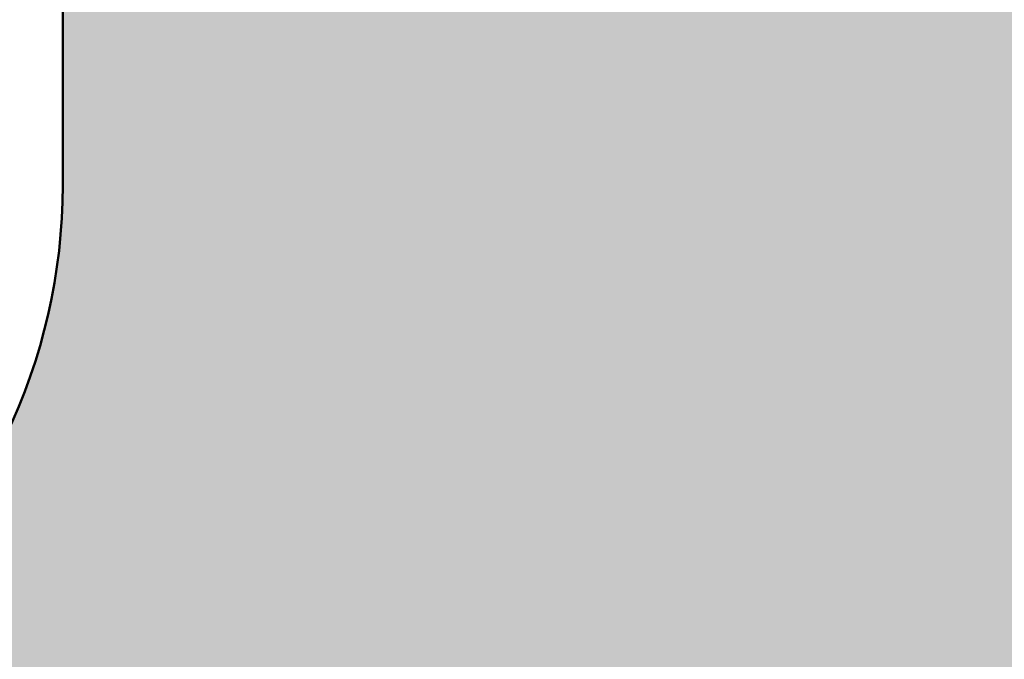
# Model space of a CAD drawing. Units: millimetres. Extents: x 0 to 2267, y 0 to 1823.
# Tile 28 of 256: x 1590 to 1675, y 1160 to 1216. Entities that reach past the tile are written whole.
import ezdxf

# ---------------------------------------------------------------- set-up
doc = ezdxf.new("R2010")
doc.units = ezdxf.units.MM
doc.header["$MEASUREMENT"] = 0
doc.layers.add('M-HATC', color=252, linetype='Continuous', lineweight=18)
doc.layers.add('M-OUTL', color=7, linetype='Continuous', lineweight=50)

msp = doc.modelspace()

# ---------------------------------------------------------------- hatches: boundary and pattern name
at = {"layer": 'M-HATC'}
h = msp.add_hatch(color=256, dxfattribs=at)
h.dxf.hatch_style = 1
h.paths.add_polyline_path([(2055.771, 1603.062), (1381.087, 1603.062), (1381.087, 1598.062), (2055.771, 1598.062)])
h.paths.add_polyline_path([(2055.771, 1598.062), (1381.087, 1598.062), (1381.087, 1593.062), (2055.771, 1593.062)])
h.paths.add_polyline_path([(2051.307, 1536.761), (1385.55, 1536.761), (1385.55, 1526.761), (1387.55, 1526.761), (1388.537, 1525.053), (1385.332, 1521.233), (1385.332, 1521.223), (2050.254, 1522.749), (2048.321, 1525.053), (2049.307, 1526.761), (2051.307, 1526.761)])
edge = h.paths.add_edge_path()
edge.add_arc((1847.535, 1379.149), 135, 222.60306, 222.89085, ccw=False)
edge.add_line((1748.166, 1287.766), (1683.092, 1287.766))
edge.add_arc((1583.724, 1379.149), 135, 317.10915, 317.39694, ccw=False)
edge.add_arc((1678.969, 1290.671), 5, 222.89085, 317.10915, ccw=False)
edge.add_arc((1774.213, 1379.149), 135, 222.60306, 222.89085, ccw=False)
edge.add_line((1674.845, 1287.766), (1609.771, 1287.766))
edge.add_arc((1510.403, 1379.149), 135, 317.10915, 317.39694, ccw=False)
edge.add_arc((1605.647, 1290.671), 5, 222.89085, 317.10915, ccw=False)
edge.add_arc((1700.892, 1379.149), 135, 222.60306, 222.89085, ccw=False)
edge.add_line((1601.524, 1287.766), (1536.45, 1287.766))
edge.add_arc((1437.081, 1379.149), 135, 317.10915, 317.39694, ccw=False)
edge.add_arc((1532.326, 1290.671), 5, 222.89085, 317.10915, ccw=False)
edge.add_arc((1627.571, 1379.149), 135, 222.60306, 222.89085, ccw=False)
edge.add_line((1528.203, 1287.766), (1505.929, 1287.766))
edge.add_spline(control_points=[(1505.929, 1287.766), (1504.262, 1287.766), (1504.262, 1282.766), (1505.929, 1282.766)], knot_values=[0, 0, 0, 0, 5, 5, 5, 5], degree=3, periodic=0)
edge.add_line((1505.929, 1282.766), (1930.929, 1282.766))
edge.add_spline(control_points=[(1930.929, 1282.766), (1932.596, 1282.766), (1932.596, 1287.766), (1930.929, 1287.766)], knot_values=[0, 0, 0, 0, 5, 5, 5, 5], degree=3, periodic=0)
edge.add_line((1930.929, 1287.766), (1903.056, 1287.766))
edge.add_arc((1803.688, 1379.149), 135, 317.10915, 317.39694, ccw=False)
edge.add_arc((1898.932, 1290.671), 5, 222.89085, 317.10915, ccw=False)
edge.add_arc((1994.177, 1379.149), 135, 222.60306, 222.89085, ccw=False)
edge.add_line((1894.809, 1287.766), (1829.735, 1287.766))
edge.add_arc((1730.366, 1379.149), 135, 317.10915, 317.39694, ccw=False)
edge.add_arc((1825.611, 1290.671), 5, 222.89085, 317.10915, ccw=False)
edge.add_arc((1920.856, 1379.149), 135, 222.60306, 222.89085, ccw=False)
edge.add_line((1821.487, 1287.766), (1756.413, 1287.766))
edge.add_arc((1657.045, 1379.149), 135, 317.10915, 317.39694, ccw=False)
edge.add_arc((1752.29, 1290.671), 5, 222.89085, 317.10915, ccw=False)
edge = h.paths.add_edge_path()
edge.add_spline(control_points=[(1843.429, 1227.247), (1845.096, 1227.247), (1845.096, 1232.247), (1843.429, 1232.247)], knot_values=[0, 0, 0, 0, 5, 5, 5, 5], degree=3, periodic=0)
edge.add_line((1843.429, 1232.247), (1593.429, 1232.247))
edge.add_spline(control_points=[(1593.429, 1232.247), (1591.762, 1232.247), (1591.762, 1227.247), (1593.429, 1227.247)], knot_values=[0, 0, 0, 0, 5, 5, 5, 5], degree=3, periodic=0)
edge.add_line((1593.429, 1227.247), (1843.429, 1227.247))
h.paths.add_polyline_path([(1905.929, 1127.417), (1530.929, 1127.417, 0.414214), (1520.929, 1117.417), (1530.929, 1117.417), (1915.929, 1117.417, 0.414214)])
edge = h.paths.add_edge_path()
edge.add_arc((1397.086, 1498.408), 12.73, 90.78215, 190.87871, ccw=False)
edge.add_line((1396.912, 1511.136), (1428.01, 1511.349))
edge.add_line((1428.01, 1511.349), (1433.01, 1511.349))
edge.add_line((1433.01, 1511.349), (1434.439, 1511.349))
edge.add_arc((1419.474, 1498.08), 20, 41.561, 74.08211)
edge.add_line((1424.959, 1517.314), (1399.935, 1517.256))
edge.add_spline(control_points=[(1399.931, 1517.256), (1399.884, 1517.213), (1399.833, 1517.169), (1399.777, 1517.124)], knot_values=[11.567499, 11.567499, 11.567499, 11.567499, 11.814249, 11.814249, 11.814249, 11.814249], degree=3, periodic=0)
edge.add_spline(control_points=[(1399.633, 1517.01), (1399.583, 1516.972), (1399.531, 1516.934), (1399.476, 1516.895)], knot_values=[11.167718, 11.167718, 11.167718, 11.167718, 11.365188, 11.365188, 11.365188, 11.365188], degree=3, periodic=0)
edge.add_spline(control_points=[(1399.34, 1516.8), (1399.151, 1516.672), (1398.938, 1516.538), (1398.704, 1516.399)], knot_values=[10.376405, 10.376405, 10.376405, 10.376405, 11.00994, 11.00994, 11.00994, 11.00994], degree=3, periodic=0)
edge.add_spline(control_points=[(1398.657, 1516.372), (1398.579, 1516.326), (1398.498, 1516.28), (1398.415, 1516.233)], knot_values=[10.125175, 10.125175, 10.125175, 10.125175, 10.334406, 10.334406, 10.334406, 10.334406], degree=3, periodic=0)
edge.add_spline(control_points=[(1398.264, 1516.149), (1398.196, 1516.111), (1398.126, 1516.073), (1398.055, 1516.035)], knot_values=[9.832246, 9.832246, 9.832246, 9.832246, 9.999658, 9.999658, 9.999658, 9.999658], degree=3, periodic=0)
edge.add_spline(control_points=[(1397.999, 1516.005), (1397.731, 1515.862), (1397.446, 1515.717), (1397.147, 1515.571)], knot_values=[9.161808, 9.161808, 9.161808, 9.161808, 9.787769, 9.787769, 9.787769, 9.787769], degree=3, periodic=0)
edge.add_spline(control_points=[(1397.147, 1515.571), (1396.842, 1515.423), (1396.522, 1515.274), (1396.191, 1515.126)], knot_values=[8.524455, 8.524455, 8.524455, 8.524455, 9.161808, 9.161808, 9.161808, 9.161808], degree=3, periodic=0)
edge.add_spline(control_points=[(1396.078, 1515.076), (1395.985, 1515.035), (1395.892, 1514.994), (1395.798, 1514.953)], knot_values=[8.275193, 8.275193, 8.275193, 8.275193, 8.451726, 8.451726, 8.451726, 8.451726], degree=3, periodic=0)
edge.add_spline(control_points=[(1395.602, 1514.869), (1395.5, 1514.826), (1395.397, 1514.782), (1395.293, 1514.739)], knot_values=[7.962917, 7.962917, 7.962917, 7.962917, 8.152764, 8.152764, 8.152764, 8.152764], degree=3, periodic=0)
edge.add_spline(control_points=[(1395.212, 1514.706), (1394.828, 1514.547), (1394.435, 1514.393), (1394.036, 1514.244)], knot_values=[7.21254, 7.21254, 7.21254, 7.21254, 7.913148, 7.913148, 7.913148, 7.913148], degree=3, periodic=0)
edge.add_spline(control_points=[(1394.036, 1514.244), (1393.708, 1514.121), (1393.375, 1514.003), (1393.043, 1513.889)], knot_values=[6.633733, 6.633733, 6.633733, 6.633733, 7.21254, 7.21254, 7.21254, 7.21254], degree=3, periodic=0)
edge.add_spline(control_points=[(1392.821, 1513.815), (1392.72, 1513.781), (1392.618, 1513.748), (1392.517, 1513.715)], knot_values=[6.328796, 6.328796, 6.328796, 6.328796, 6.505493, 6.505493, 6.505493, 6.505493], degree=3, periodic=0)
edge.add_spline(control_points=[(1392.517, 1513.715), (1392.319, 1513.652), (1392.121, 1513.59), (1391.924, 1513.531)], knot_values=[5.984605, 5.984605, 5.984605, 5.984605, 6.328796, 6.328796, 6.328796, 6.328796], degree=3, periodic=0)
edge.add_spline(control_points=[(1391.792, 1513.491), (1391.312, 1513.35), (1390.838, 1513.224), (1390.378, 1513.117)], knot_values=[5.066697, 5.066697, 5.066697, 5.066697, 5.907055, 5.907055, 5.907055, 5.907055], degree=3, periodic=0)
edge.add_spline(control_points=[(1390.378, 1513.117), (1390.18, 1513.071), (1389.984, 1513.028), (1389.791, 1512.99)], knot_values=[4.70367, 4.70367, 4.70367, 4.70367, 5.066695, 5.066695, 5.066695, 5.066695], degree=3, periodic=0)
edge.add_spline(control_points=[(1389.422, 1512.92), (1389.246, 1512.889), (1389.073, 1512.862), (1388.904, 1512.838)], knot_values=[4.130571, 4.130571, 4.130571, 4.130571, 4.469816, 4.469816, 4.469816, 4.469816], degree=3, periodic=0)
edge.add_spline(control_points=[(1388.904, 1512.838), (1388.591, 1512.795), (1388.291, 1512.764), (1388.007, 1512.749)], knot_values=[3.504031, 3.504031, 3.504031, 3.504031, 4.130571, 4.130571, 4.130571, 4.130571], degree=3, periodic=0)
edge.add_spline(control_points=[(1387.936, 1512.746), (1387.854, 1512.742), (1387.773, 1512.74), (1387.694, 1512.739)], knot_values=[3.268866, 3.268866, 3.268866, 3.268866, 3.451164, 3.451164, 3.451164, 3.451164], degree=3, periodic=0)
edge.add_spline(control_points=[(1387.335, 1512.744), (1387.208, 1512.75), (1387.085, 1512.76), (1386.967, 1512.774)], knot_values=[2.670686, 2.670686, 2.670686, 2.670686, 2.984, 2.984, 2.984, 2.984], degree=3, periodic=0)
edge.add_spline(control_points=[(1386.833, 1512.792), (1386.821, 1512.794), (1386.809, 1512.796), (1386.797, 1512.798)], knot_values=[2.516981, 2.516981, 2.516981, 2.516981, 2.549528, 2.549528, 2.549528, 2.549528], degree=3, periodic=0)
edge.add_spline(control_points=[(1386.453, 1512.873), (1386.426, 1512.881), (1386.399, 1512.889), (1386.373, 1512.897)], knot_values=[2.095869, 2.095869, 2.095869, 2.095869, 2.17941, 2.17941, 2.17941, 2.17941], degree=3, periodic=0)
edge.add_spline(control_points=[(1386.069, 1513.019), (1386.063, 1513.022), (1386.058, 1513.025), (1386.052, 1513.028)], knot_values=[1.72453, 1.72453, 1.72453, 1.72453, 1.745933, 1.745933, 1.745933, 1.745933], degree=3, periodic=0)
edge.add_arc((1399.474, 1498.08), 20, 131.82432, 180)
edge.add_arc((1630.334, 1505.548), 250.971, 181.70518, 236.42798)
edge.add_arc((1605.34, 1483.304), 218.782, 238.66083, 243.34961)
edge.add_arc((1647.091, 1510.359), 262.899, 183.12984, 237.85344, ccw=False)
h.paths.add_polyline_path([(1406.537, 1391.964, 0.149382), (1491.551, 1296.442, -0.129517)], flags=17)
edge = h.paths.add_edge_path()
edge.add_arc((2037.384, 1498.08), 20, 0, 48.26587)
edge.add_spline(control_points=[(2050.697, 1513.005), (2050.651, 1512.985), (2050.603, 1512.966), (2050.554, 1512.948)], knot_values=[1.835652, 1.835652, 1.835652, 1.835652, 2.000781, 2.000781, 2.000781, 2.000781], degree=3, periodic=0)
edge.add_spline(control_points=[(2050.462, 1512.917), (2050.479, 1512.922), (2050.496, 1512.928), (2050.513, 1512.934)], knot_values=[2.045477, 2.045477, 2.045477, 2.045477, 2.101389, 2.101389, 2.101389, 2.101389], degree=3, periodic=0)
edge.add_spline(control_points=[(2050.129, 1512.834), (2050.198, 1512.847), (2050.266, 1512.862), (2050.331, 1512.879)], knot_values=[2.237629, 2.237629, 2.237629, 2.237629, 2.435841, 2.435841, 2.435841, 2.435841], degree=3, periodic=0)
edge.add_spline(control_points=[(2050.095, 1512.828), (2050.106, 1512.83), (2050.118, 1512.832), (2050.129, 1512.834)], knot_values=[2.435841, 2.435841, 2.435841, 2.435841, 2.468321, 2.468321, 2.468321, 2.468321], degree=3, periodic=0)
edge.add_spline(control_points=[(2049.784, 1512.785), (2049.855, 1512.792), (2049.924, 1512.801), (2049.992, 1512.811)], knot_values=[2.563852, 2.563852, 2.563852, 2.563852, 2.748541, 2.748541, 2.748541, 2.748541], degree=3, periodic=0)
edge.add_spline(control_points=[(2049.405, 1512.762), (2049.536, 1512.765), (2049.663, 1512.773), (2049.784, 1512.785)], knot_values=[2.748541, 2.748541, 2.748541, 2.748541, 3.064882, 3.064882, 3.064882, 3.064882], degree=3, periodic=0)
edge.add_spline(control_points=[(2049.17, 1512.76), (2049.234, 1512.759), (2049.297, 1512.759), (2049.358, 1512.761)], knot_values=[3.102309, 3.102309, 3.102309, 3.102309, 3.2503, 3.2503, 3.2503, 3.2503], degree=3, periodic=0)
edge.add_spline(control_points=[(2048.857, 1512.769), (2048.964, 1512.764), (2049.068, 1512.761), (2049.17, 1512.76)], knot_values=[3.2503, 3.2503, 3.2503, 3.2503, 3.486069, 3.486069, 3.486069, 3.486069], degree=3, periodic=0)
edge.add_spline(control_points=[(2048.692, 1512.779), (2048.373, 1512.801), (2048.035, 1512.841), (2047.682, 1512.897)], knot_values=[3.606429, 3.606429, 3.606429, 3.606429, 4.2989, 4.2989, 4.2989, 4.2989], degree=3, periodic=0)
edge.add_spline(control_points=[(2047.682, 1512.897), (2047.546, 1512.919), (2047.408, 1512.942), (2047.268, 1512.969)], knot_values=[4.2989, 4.2989, 4.2989, 4.2989, 4.565769, 4.565769, 4.565769, 4.565769], degree=3, periodic=0)
edge.add_spline(control_points=[(2047.268, 1512.969), (2047.145, 1512.991), (2047.021, 1513.016), (2046.895, 1513.042)], knot_values=[4.565769, 4.565769, 4.565769, 4.565769, 4.799971, 4.799971, 4.799971, 4.799971], degree=3, periodic=0)
edge.add_spline(control_points=[(2046.895, 1513.042), (2046.529, 1513.119), (2046.151, 1513.209), (2045.768, 1513.311)], knot_values=[4.799971, 4.799971, 4.799971, 4.799971, 5.483718, 5.483718, 5.483718, 5.483718], degree=3, periodic=0)
edge.add_spline(control_points=[(2045.768, 1513.311), (2045.372, 1513.415), (2044.97, 1513.532), (2044.566, 1513.659)], knot_values=[5.483718, 5.483718, 5.483718, 5.483718, 6.187866, 6.187866, 6.187866, 6.187866], degree=3, periodic=0)
edge.add_spline(control_points=[(2044.566, 1513.659), (2044.415, 1513.706), (2044.263, 1513.755), (2044.112, 1513.805)], knot_values=[6.187866, 6.187866, 6.187866, 6.187866, 6.451551, 6.451551, 6.451551, 6.451551], degree=3, periodic=0)
edge.add_spline(control_points=[(2044.112, 1513.805), (2043.997, 1513.843), (2043.882, 1513.881), (2043.767, 1513.92)], knot_values=[6.451551, 6.451551, 6.451551, 6.451551, 6.651434, 6.651434, 6.651434, 6.651434], degree=3, periodic=0)
edge.add_spline(control_points=[(2043.767, 1513.92), (2043.372, 1514.055), (2042.977, 1514.198), (2042.589, 1514.346)], knot_values=[6.651434, 6.651434, 6.651434, 6.651434, 7.338879, 7.338879, 7.338879, 7.338879], degree=3, periodic=0)
edge.add_spline(control_points=[(2042.589, 1514.346), (2042.164, 1514.507), (2041.746, 1514.675), (2041.341, 1514.846)], knot_values=[7.338879, 7.338879, 7.338879, 7.338879, 8.089209, 8.089209, 8.089209, 8.089209], degree=3, periodic=0)
edge.add_spline(control_points=[(2041.341, 1514.846), (2041.103, 1514.946), (2040.869, 1515.048), (2040.64, 1515.15)], knot_values=[8.089209, 8.089209, 8.089209, 8.089209, 8.529587, 8.529587, 8.529587, 8.529587], degree=3, periodic=0)
edge.add_spline(control_points=[(2040.51, 1515.209), (2040.082, 1515.402), (2039.675, 1515.597), (2039.295, 1515.789)], knot_values=[8.613818, 8.613818, 8.613818, 8.613818, 9.44571, 9.44571, 9.44571, 9.44571], degree=3, periodic=0)
edge.add_spline(control_points=[(2039.295, 1515.789), (2039.062, 1515.907), (2038.839, 1516.025), (2038.629, 1516.14)], knot_values=[9.44571, 9.44571, 9.44571, 9.44571, 9.956404, 9.956404, 9.956404, 9.956404], degree=3, periodic=0)
edge.add_spline(control_points=[(2038.629, 1516.14), (2038.519, 1516.2), (2038.412, 1516.26), (2038.309, 1516.319)], knot_values=[9.956404, 9.956404, 9.956404, 9.956404, 10.223542, 10.223542, 10.223542, 10.223542], degree=3, periodic=0)
edge.add_spline(control_points=[(2038.309, 1516.319), (2038.214, 1516.374), (2038.122, 1516.428), (2038.033, 1516.481)], knot_values=[10.223542, 10.223542, 10.223542, 10.223542, 10.47051, 10.47051, 10.47051, 10.47051], degree=3, periodic=0)
edge.add_spline(control_points=[(2038.033, 1516.481), (2037.786, 1516.63), (2037.564, 1516.773), (2037.372, 1516.909)], knot_values=[10.47051, 10.47051, 10.47051, 10.47051, 11.15767, 11.15767, 11.15767, 11.15767], degree=3, periodic=0)
edge.add_spline(control_points=[(2037.372, 1516.909), (2037.279, 1516.975), (2037.193, 1517.04), (2037.114, 1517.102)], knot_values=[11.15767, 11.15767, 11.15767, 11.15767, 11.49227, 11.49227, 11.49227, 11.49227], degree=3, periodic=0)
edge.add_spline(control_points=[(2036.856, 1517.326), (2036.915, 1517.269), (2036.981, 1517.21), (2037.056, 1517.149)], knot_values=[11.577341, 11.577341, 11.577341, 11.577341, 11.91035, 11.91035, 11.91035, 11.91035], degree=3, periodic=0)
edge.add_spline(control_points=[(2036.807, 1517.375), (2036.823, 1517.359), (2036.839, 1517.342), (2036.856, 1517.326)], knot_values=[11.91035, 11.91035, 11.91035, 11.91035, 12.007402, 12.007402, 12.007402, 12.007402], degree=3, periodic=0)
edge.add_spline(control_points=[(2036.702, 1517.494), (2036.71, 1517.483), (2036.72, 1517.472), (2036.729, 1517.461)], knot_values=[12.184155, 12.184155, 12.184155, 12.184155, 12.255409, 12.255409, 12.255409, 12.255409], degree=3, periodic=0)
edge.add_spline(control_points=[(2036.616, 1517.621), (2036.62, 1517.613), (2036.624, 1517.606), (2036.629, 1517.598)], knot_values=[12.487913, 12.487913, 12.487913, 12.487913, 12.541035, 12.541035, 12.541035, 12.541035], degree=3, periodic=0)
edge.add_spline(control_points=[(2036.563, 1517.786), (2036.564, 1517.779), (2036.564, 1517.773), (2036.565, 1517.766)], knot_values=[12.911761, 12.911761, 12.911761, 12.911761, 12.968286, 12.968286, 12.968286, 12.968286], degree=3, periodic=0)
edge.add_spline(control_points=[(2036.617, 1517.93), (2036.612, 1517.926), (2036.609, 1517.921), (2036.605, 1517.916)], knot_values=[13.382527, 13.382527, 13.382527, 13.382527, 13.433791, 13.433791, 13.433791, 13.433791], degree=3, periodic=0)
edge.add_spline(control_points=[(2036.749, 1518.017), (2036.736, 1518.012), (2036.724, 1518.006), (2036.712, 1518)], knot_values=[13.726299, 13.726299, 13.726299, 13.726299, 13.809928, 13.809928, 13.809928, 13.809928], degree=3, periodic=0)
edge.add_spline(control_points=[(2036.86, 1518.053), (2036.839, 1518.047), (2036.818, 1518.042), (2036.799, 1518.035)], knot_values=[13.910887, 13.910887, 13.910887, 13.910887, 14.02153, 14.02153, 14.02153, 14.02153], degree=3, periodic=0)
edge.add_line((2036.964, 1518.08), (2032.384, 1518.08))
edge.add_line((2032.384, 1518.08), (2027.384, 1518.08))
edge.add_line((2027.384, 1518.08), (2022.384, 1518.08))
edge.add_line((2022.384, 1518.08), (2017.384, 1518.08))
edge.add_arc((2017.384, 1498.08), 20, 90, 138.439)
edge.add_line((2002.419, 1511.349), (2003.848, 1511.349))
edge.add_line((2003.848, 1511.349), (2008.848, 1511.349))
edge.add_line((2008.848, 1511.349), (2039.772, 1511.138))
edge.add_arc((2039.772, 1498.408), 12.73, -10.87871, 90, ccw=False)
edge.add_arc((1789.767, 1510.359), 262.899, 302.14656, 356.87016, ccw=False)
edge.add_arc((1831.518, 1483.304), 218.782, 296.65039, 301.33917)
edge.add_arc((1806.524, 1505.548), 250.971, 303.57202, 358.29482)
h.paths.add_polyline_path([(2030.321, 1391.964, -0.129517), (1945.307, 1296.442, 0.149382)], flags=17)
edge = h.paths.add_edge_path()
edge.add_spline(control_points=[(2037.246, 1518.082), (2037.29, 1518.081), (2037.336, 1518.08), (2037.384, 1518.08)], knot_values=[0.000012, 0.000012, 0.000012, 0.000012, 0.144754, 0.144754, 0.144754, 0.144754], degree=3, periodic=0)
edge.add_line((2037.336, 1518.08), (2037.01, 1518.08))
edge.add_spline(control_points=[(2037.01, 1518.08), (2036.982, 1518.077), (2036.956, 1518.073), (2036.931, 1518.068)], knot_values=[14.13465, 14.13465, 14.13465, 14.13465, 14.247197, 14.247197, 14.247197, 14.247197], degree=3, periodic=0)
edge.add_spline(control_points=[(2036.931, 1518.068), (2036.928, 1518.067), (2036.924, 1518.067), (2036.921, 1518.066)], knot_values=[14.118315, 14.118315, 14.118315, 14.118315, 14.13465, 14.13465, 14.13465, 14.13465], degree=3, periodic=0)
edge.add_spline(control_points=[(2036.921, 1518.066), (2036.912, 1518.064), (2036.903, 1518.063), (2036.895, 1518.061)], knot_values=[14.078086, 14.078086, 14.078086, 14.078086, 14.118315, 14.118315, 14.118315, 14.118315], degree=3, periodic=0)
edge.add_spline(control_points=[(2036.895, 1518.061), (2036.883, 1518.058), (2036.872, 1518.056), (2036.86, 1518.053)], knot_values=[14.02153, 14.02153, 14.02153, 14.02153, 14.078086, 14.078086, 14.078086, 14.078086], degree=3, periodic=0)
edge.add_spline(control_points=[(2036.86, 1518.053), (2036.839, 1518.047), (2036.818, 1518.042), (2036.799, 1518.035)], knot_values=[13.910887, 13.910887, 13.910887, 13.910887, 14.02153, 14.02153, 14.02153, 14.02153], degree=3, periodic=0)
edge.add_spline(control_points=[(2036.799, 1518.035), (2036.798, 1518.035), (2036.797, 1518.035), (2036.797, 1518.035)], knot_values=[13.906906, 13.906906, 13.906906, 13.906906, 13.910887, 13.910887, 13.910887, 13.910887], degree=3, periodic=0)
edge.add_spline(control_points=[(2036.797, 1518.035), (2036.788, 1518.032), (2036.78, 1518.029), (2036.772, 1518.026)], knot_values=[13.857826, 13.857826, 13.857826, 13.857826, 13.906906, 13.906906, 13.906906, 13.906906], degree=3, periodic=0)
edge.add_spline(control_points=[(2036.772, 1518.026), (2036.764, 1518.023), (2036.756, 1518.02), (2036.749, 1518.017)], knot_values=[13.809928, 13.809928, 13.809928, 13.809928, 13.857826, 13.857826, 13.857826, 13.857826], degree=3, periodic=0)
edge.add_spline(control_points=[(2036.749, 1518.017), (2036.736, 1518.012), (2036.724, 1518.006), (2036.712, 1518)], knot_values=[13.726299, 13.726299, 13.726299, 13.726299, 13.809928, 13.809928, 13.809928, 13.809928], degree=3, periodic=0)
edge.add_spline(control_points=[(2036.712, 1518), (2036.712, 1518), (2036.712, 1518), (2036.711, 1518)], knot_values=[13.723993, 13.723993, 13.723993, 13.723993, 13.726299, 13.726299, 13.726299, 13.726299], degree=3, periodic=0)
edge.add_spline(control_points=[(2036.711, 1518), (2036.706, 1517.997), (2036.701, 1517.994), (2036.696, 1517.992)], knot_values=[13.686536, 13.686536, 13.686536, 13.686536, 13.723993, 13.723993, 13.723993, 13.723993], degree=3, periodic=0)
edge.add_spline(control_points=[(2036.696, 1517.992), (2036.692, 1517.989), (2036.687, 1517.987), (2036.683, 1517.984)], knot_values=[13.651251, 13.651251, 13.651251, 13.651251, 13.686536, 13.686536, 13.686536, 13.686536], degree=3, periodic=0)
edge.add_spline(control_points=[(2036.683, 1517.984), (2036.676, 1517.98), (2036.67, 1517.976), (2036.664, 1517.971)], knot_values=[13.596804, 13.596804, 13.596804, 13.596804, 13.651251, 13.651251, 13.651251, 13.651251], degree=3, periodic=0)
edge.add_spline(control_points=[(2036.664, 1517.971), (2036.664, 1517.971), (2036.663, 1517.971), (2036.663, 1517.971)], knot_values=[13.593956, 13.593956, 13.593956, 13.593956, 13.596804, 13.596804, 13.596804, 13.596804], degree=3, periodic=0)
edge.add_spline(control_points=[(2036.663, 1517.971), (2036.66, 1517.969), (2036.658, 1517.967), (2036.655, 1517.965)], knot_values=[13.570322, 13.570322, 13.570322, 13.570322, 13.593956, 13.593956, 13.593956, 13.593956], degree=3, periodic=0)
edge.add_spline(control_points=[(2036.655, 1517.965), (2036.653, 1517.963), (2036.65, 1517.961), (2036.647, 1517.959)], knot_values=[13.545477, 13.545477, 13.545477, 13.545477, 13.570322, 13.570322, 13.570322, 13.570322], degree=3, periodic=0)
edge.add_spline(control_points=[(2036.647, 1517.959), (2036.647, 1517.959), (2036.647, 1517.959), (2036.647, 1517.959)], knot_values=[13.543931, 13.543931, 13.543931, 13.543931, 13.545477, 13.545477, 13.545477, 13.545477], degree=3, periodic=0)
edge.add_spline(control_points=[(2036.647, 1517.959), (2036.641, 1517.954), (2036.636, 1517.949), (2036.631, 1517.945)], knot_values=[13.488237, 13.488237, 13.488237, 13.488237, 13.543931, 13.543931, 13.543931, 13.543931], degree=3, periodic=0)
edge.add_spline(control_points=[(2036.631, 1517.945), (2036.628, 1517.942), (2036.626, 1517.94), (2036.623, 1517.937)], knot_values=[13.460307, 13.460307, 13.460307, 13.460307, 13.488237, 13.488237, 13.488237, 13.488237], degree=3, periodic=0)
edge.add_spline(control_points=[(2036.623, 1517.937), (2036.622, 1517.936), (2036.62, 1517.934), (2036.618, 1517.932)], knot_values=[13.439712, 13.439712, 13.439712, 13.439712, 13.460307, 13.460307, 13.460307, 13.460307], degree=3, periodic=0)
edge.add_spline(control_points=[(2036.618, 1517.932), (2036.618, 1517.931), (2036.617, 1517.931), (2036.617, 1517.93)], knot_values=[13.433791, 13.433791, 13.433791, 13.433791, 13.439712, 13.439712, 13.439712, 13.439712], degree=3, periodic=0)
edge.add_spline(control_points=[(2036.617, 1517.93), (2036.612, 1517.926), (2036.609, 1517.921), (2036.605, 1517.916)], knot_values=[13.382527, 13.382527, 13.382527, 13.382527, 13.433791, 13.433791, 13.433791, 13.433791], degree=3, periodic=0)
edge.add_spline(control_points=[(2036.605, 1517.916), (2036.603, 1517.913), (2036.6, 1517.91), (2036.598, 1517.907)], knot_values=[13.350017, 13.350017, 13.350017, 13.350017, 13.382527, 13.382527, 13.382527, 13.382527], degree=3, periodic=0)
edge.add_spline(control_points=[(2036.598, 1517.907), (2036.597, 1517.906), (2036.596, 1517.904), (2036.595, 1517.903)], knot_values=[13.333922, 13.333922, 13.333922, 13.333922, 13.350017, 13.350017, 13.350017, 13.350017], degree=3, periodic=0)
edge.add_spline(control_points=[(2036.595, 1517.903), (2036.595, 1517.902), (2036.594, 1517.901), (2036.593, 1517.9)], knot_values=[13.323828, 13.323828, 13.323828, 13.323828, 13.333922, 13.333922, 13.333922, 13.333922], degree=3, periodic=0)
edge.add_spline(control_points=[(2036.593, 1517.9), (2036.59, 1517.895), (2036.588, 1517.891), (2036.585, 1517.886)], knot_values=[13.277545, 13.277545, 13.277545, 13.277545, 13.323828, 13.323828, 13.323828, 13.323828], degree=3, periodic=0)
edge.add_spline(control_points=[(2036.585, 1517.886), (2036.584, 1517.883), (2036.582, 1517.879), (2036.58, 1517.875)], knot_values=[13.240119, 13.240119, 13.240119, 13.240119, 13.277545, 13.277545, 13.277545, 13.277545], degree=3, periodic=0)
edge.add_spline(control_points=[(2036.58, 1517.875), (2036.58, 1517.874), (2036.579, 1517.873), (2036.578, 1517.872)], knot_values=[13.228211, 13.228211, 13.228211, 13.228211, 13.240119, 13.240119, 13.240119, 13.240119], degree=3, periodic=0)
edge.add_spline(control_points=[(2036.578, 1517.872), (2036.578, 1517.87), (2036.577, 1517.869), (2036.577, 1517.868)], knot_values=[13.215717, 13.215717, 13.215717, 13.215717, 13.228211, 13.228211, 13.228211, 13.228211], degree=3, periodic=0)
edge.add_spline(control_points=[(2036.577, 1517.868), (2036.575, 1517.864), (2036.574, 1517.86), (2036.573, 1517.857)], knot_values=[13.179847, 13.179847, 13.179847, 13.179847, 13.215717, 13.215717, 13.215717, 13.215717], degree=3, periodic=0)
edge.add_spline(control_points=[(2036.573, 1517.857), (2036.571, 1517.851), (2036.57, 1517.846), (2036.569, 1517.841)], knot_values=[13.132017, 13.132017, 13.132017, 13.132017, 13.179847, 13.179847, 13.179847, 13.179847], degree=3, periodic=0)
edge.add_spline(control_points=[(2036.569, 1517.841), (2036.568, 1517.84), (2036.568, 1517.839), (2036.568, 1517.838)], knot_values=[13.122482, 13.122482, 13.122482, 13.122482, 13.132017, 13.132017, 13.132017, 13.132017], degree=3, periodic=0)
edge.add_spline(control_points=[(2036.568, 1517.838), (2036.568, 1517.836), (2036.567, 1517.835), (2036.567, 1517.833)], knot_values=[13.105592, 13.105592, 13.105592, 13.105592, 13.122482, 13.122482, 13.122482, 13.122482], degree=3, periodic=0)
edge.add_spline(control_points=[(2036.567, 1517.833), (2036.566, 1517.829), (2036.566, 1517.826), (2036.565, 1517.822)], knot_values=[13.074063, 13.074063, 13.074063, 13.074063, 13.105592, 13.105592, 13.105592, 13.105592], degree=3, periodic=0)
edge.add_spline(control_points=[(2036.565, 1517.822), (2036.565, 1517.822), (2036.565, 1517.822), (2036.565, 1517.822)], knot_values=[13.074043, 13.074043, 13.074043, 13.074043, 13.074063, 13.074063, 13.074063, 13.074063], degree=3, periodic=0)
edge.add_spline(control_points=[(2036.565, 1517.822), (2036.564, 1517.816), (2036.564, 1517.811), (2036.564, 1517.805)], knot_values=[13.021884, 13.021884, 13.021884, 13.021884, 13.074043, 13.074043, 13.074043, 13.074043], degree=3, periodic=0)
edge.add_spline(control_points=[(2036.564, 1517.805), (2036.564, 1517.804), (2036.564, 1517.803), (2036.564, 1517.803)], knot_values=[13.01674, 13.01674, 13.01674, 13.01674, 13.021884, 13.021884, 13.021884, 13.021884], degree=3, periodic=0)
edge.add_spline(control_points=[(2036.564, 1517.803), (2036.563, 1517.801), (2036.563, 1517.798), (2036.563, 1517.796)], knot_values=[12.996438, 12.996438, 12.996438, 12.996438, 13.01674, 13.01674, 13.01674, 13.01674], degree=3, periodic=0)
edge.add_spline(control_points=[(2036.563, 1517.796), (2036.563, 1517.793), (2036.563, 1517.789), (2036.563, 1517.786)], knot_values=[12.968286, 12.968286, 12.968286, 12.968286, 12.996438, 12.996438, 12.996438, 12.996438], degree=3, periodic=0)
edge.add_spline(control_points=[(2036.563, 1517.786), (2036.564, 1517.779), (2036.564, 1517.773), (2036.565, 1517.766)], knot_values=[12.911761, 12.911761, 12.911761, 12.911761, 12.968286, 12.968286, 12.968286, 12.968286], degree=3, periodic=0)
edge.add_spline(control_points=[(2036.565, 1517.766), (2036.565, 1517.766), (2036.565, 1517.766), (2036.565, 1517.766)], knot_values=[12.911017, 12.911017, 12.911017, 12.911017, 12.911761, 12.911761, 12.911761, 12.911761], degree=3, periodic=0)
edge.add_spline(control_points=[(2036.565, 1517.766), (2036.565, 1517.762), (2036.566, 1517.759), (2036.566, 1517.756)], knot_values=[12.88528, 12.88528, 12.88528, 12.88528, 12.911017, 12.911017, 12.911017, 12.911017], degree=3, periodic=0)
edge.add_spline(control_points=[(2036.566, 1517.756), (2036.567, 1517.753), (2036.567, 1517.751), (2036.568, 1517.748)], knot_values=[12.862519, 12.862519, 12.862519, 12.862519, 12.88528, 12.88528, 12.88528, 12.88528], degree=3, periodic=0)
edge.add_spline(control_points=[(2036.568, 1517.748), (2036.568, 1517.747), (2036.568, 1517.747), (2036.568, 1517.746)], knot_values=[12.858885, 12.858885, 12.858885, 12.858885, 12.862519, 12.862519, 12.862519, 12.862519], degree=3, periodic=0)
edge.add_spline(control_points=[(2036.568, 1517.746), (2036.569, 1517.74), (2036.571, 1517.733), (2036.572, 1517.726)], knot_values=[12.8053, 12.8053, 12.8053, 12.8053, 12.858885, 12.858885, 12.858885, 12.858885], degree=3, periodic=0)
edge.add_spline(control_points=[(2036.572, 1517.726), (2036.573, 1517.723), (2036.574, 1517.719), (2036.576, 1517.715)], knot_values=[12.775176, 12.775176, 12.775176, 12.775176, 12.8053, 12.8053, 12.8053, 12.8053], degree=3, periodic=0)
edge.add_spline(control_points=[(2036.576, 1517.715), (2036.576, 1517.713), (2036.577, 1517.71), (2036.578, 1517.708)], knot_values=[12.756759, 12.756759, 12.756759, 12.756759, 12.775176, 12.775176, 12.775176, 12.775176], degree=3, periodic=0)
edge.add_spline(control_points=[(2036.578, 1517.708), (2036.578, 1517.707), (2036.578, 1517.706), (2036.579, 1517.705)], knot_values=[12.748742, 12.748742, 12.748742, 12.748742, 12.756759, 12.756759, 12.756759, 12.756759], degree=3, periodic=0)
edge.add_spline(control_points=[(2036.579, 1517.705), (2036.581, 1517.698), (2036.583, 1517.692), (2036.586, 1517.685)], knot_values=[12.69959, 12.69959, 12.69959, 12.69959, 12.748742, 12.748742, 12.748742, 12.748742], degree=3, periodic=0)
edge.add_spline(control_points=[(2036.586, 1517.685), (2036.588, 1517.68), (2036.59, 1517.675), (2036.592, 1517.669)], knot_values=[12.659038, 12.659038, 12.659038, 12.659038, 12.69959, 12.69959, 12.69959, 12.69959], degree=3, periodic=0)
edge.add_spline(control_points=[(2036.592, 1517.669), (2036.594, 1517.665), (2036.596, 1517.66), (2036.598, 1517.656)], knot_values=[12.626806, 12.626806, 12.626806, 12.626806, 12.659038, 12.659038, 12.659038, 12.659038], degree=3, periodic=0)
edge.add_spline(control_points=[(2036.598, 1517.656), (2036.598, 1517.655), (2036.599, 1517.654), (2036.599, 1517.653)], knot_values=[12.619394, 12.619394, 12.619394, 12.619394, 12.626806, 12.626806, 12.626806, 12.626806], degree=3, periodic=0)
edge.add_spline(control_points=[(2036.599, 1517.653), (2036.604, 1517.642), (2036.61, 1517.632), (2036.616, 1517.621)], knot_values=[12.541039, 12.541039, 12.541039, 12.541039, 12.619394, 12.619394, 12.619394, 12.619394], degree=3, periodic=0)
edge.add_spline(control_points=[(2036.616, 1517.621), (2036.616, 1517.621), (2036.616, 1517.621), (2036.616, 1517.621)], knot_values=[12.541035, 12.541035, 12.541035, 12.541035, 12.541039, 12.541039, 12.541039, 12.541039], degree=3, periodic=0)
edge.add_spline(control_points=[(2036.616, 1517.621), (2036.62, 1517.613), (2036.624, 1517.606), (2036.629, 1517.598)], knot_values=[12.487913, 12.487913, 12.487913, 12.487913, 12.541035, 12.541035, 12.541035, 12.541035], degree=3, periodic=0)
edge.add_spline(control_points=[(2036.629, 1517.598), (2036.633, 1517.592), (2036.637, 1517.585), (2036.641, 1517.579)], knot_values=[12.443982, 12.443982, 12.443982, 12.443982, 12.487913, 12.487913, 12.487913, 12.487913], degree=3, periodic=0)
edge.add_spline(control_points=[(2036.641, 1517.579), (2036.641, 1517.578), (2036.642, 1517.576), (2036.643, 1517.575)], knot_values=[12.434996, 12.434996, 12.434996, 12.434996, 12.443982, 12.443982, 12.443982, 12.443982], degree=3, periodic=0)
edge.add_spline(control_points=[(2036.643, 1517.575), (2036.653, 1517.56), (2036.664, 1517.544), (2036.676, 1517.528)], knot_values=[12.329647, 12.329647, 12.329647, 12.329647, 12.434996, 12.434996, 12.434996, 12.434996], degree=3, periodic=0)
edge.add_spline(control_points=[(2036.676, 1517.528), (2036.684, 1517.517), (2036.693, 1517.505), (2036.702, 1517.494)], knot_values=[12.255409, 12.255409, 12.255409, 12.255409, 12.329647, 12.329647, 12.329647, 12.329647], degree=3, periodic=0)
edge.add_spline(control_points=[(2036.702, 1517.494), (2036.71, 1517.483), (2036.72, 1517.472), (2036.729, 1517.461)], knot_values=[12.184155, 12.184155, 12.184155, 12.184155, 12.255409, 12.255409, 12.255409, 12.255409], degree=3, periodic=0)
edge.add_spline(control_points=[(2036.729, 1517.461), (2036.744, 1517.444), (2036.759, 1517.426), (2036.775, 1517.409)], knot_values=[12.075961, 12.075961, 12.075961, 12.075961, 12.184155, 12.184155, 12.184155, 12.184155], degree=3, periodic=0)
edge.add_spline(control_points=[(2036.775, 1517.409), (2036.776, 1517.407), (2036.777, 1517.406), (2036.778, 1517.405)], knot_values=[12.069502, 12.069502, 12.069502, 12.069502, 12.075961, 12.075961, 12.075961, 12.075961], degree=3, periodic=0)
edge.add_spline(control_points=[(2036.778, 1517.405), (2036.788, 1517.395), (2036.797, 1517.385), (2036.807, 1517.375)], knot_values=[12.007402, 12.007402, 12.007402, 12.007402, 12.069502, 12.069502, 12.069502, 12.069502], degree=3, periodic=0)
edge.add_spline(control_points=[(2036.807, 1517.375), (2036.823, 1517.359), (2036.839, 1517.342), (2036.856, 1517.326)], knot_values=[11.91035, 11.91035, 11.91035, 11.91035, 12.007402, 12.007402, 12.007402, 12.007402], degree=3, periodic=0)
edge.add_spline(control_points=[(2036.856, 1517.326), (2036.915, 1517.269), (2036.981, 1517.21), (2037.056, 1517.149)], knot_values=[11.577341, 11.577341, 11.577341, 11.577341, 11.91035, 11.91035, 11.91035, 11.91035], degree=3, periodic=0)
edge.add_spline(control_points=[(2037.056, 1517.149), (2037.075, 1517.134), (2037.094, 1517.118), (2037.114, 1517.102)], knot_values=[11.49227, 11.49227, 11.49227, 11.49227, 11.577341, 11.577341, 11.577341, 11.577341], degree=3, periodic=0)
edge.add_spline(control_points=[(2037.114, 1517.102), (2037.193, 1517.04), (2037.279, 1516.975), (2037.372, 1516.909)], knot_values=[11.15767, 11.15767, 11.15767, 11.15767, 11.49227, 11.49227, 11.49227, 11.49227], degree=3, periodic=0)
edge.add_spline(control_points=[(2037.372, 1516.909), (2037.564, 1516.773), (2037.786, 1516.63), (2038.033, 1516.481)], knot_values=[10.47051, 10.47051, 10.47051, 10.47051, 11.15767, 11.15767, 11.15767, 11.15767], degree=3, periodic=0)
edge.add_spline(control_points=[(2038.033, 1516.481), (2038.122, 1516.428), (2038.214, 1516.374), (2038.309, 1516.319)], knot_values=[10.223542, 10.223542, 10.223542, 10.223542, 10.47051, 10.47051, 10.47051, 10.47051], degree=3, periodic=0)
edge.add_spline(control_points=[(2038.309, 1516.319), (2038.412, 1516.26), (2038.519, 1516.2), (2038.629, 1516.14)], knot_values=[9.956404, 9.956404, 9.956404, 9.956404, 10.223542, 10.223542, 10.223542, 10.223542], degree=3, periodic=0)
edge.add_spline(control_points=[(2038.629, 1516.14), (2038.839, 1516.025), (2039.062, 1515.907), (2039.295, 1515.789)], knot_values=[9.44571, 9.44571, 9.44571, 9.44571, 9.956404, 9.956404, 9.956404, 9.956404], degree=3, periodic=0)
edge.add_spline(control_points=[(2039.295, 1515.789), (2039.675, 1515.597), (2040.082, 1515.402), (2040.51, 1515.209)], knot_values=[8.613818, 8.613818, 8.613818, 8.613818, 9.44571, 9.44571, 9.44571, 9.44571], degree=3, periodic=0)
edge.add_spline(control_points=[(2040.51, 1515.209), (2040.553, 1515.189), (2040.597, 1515.17), (2040.64, 1515.15)], knot_values=[8.529587, 8.529587, 8.529587, 8.529587, 8.613818, 8.613818, 8.613818, 8.613818], degree=3, periodic=0)
edge.add_spline(control_points=[(2040.64, 1515.15), (2040.869, 1515.048), (2041.103, 1514.946), (2041.341, 1514.846)], knot_values=[8.089209, 8.089209, 8.089209, 8.089209, 8.529587, 8.529587, 8.529587, 8.529587], degree=3, periodic=0)
edge.add_spline(control_points=[(2041.341, 1514.846), (2041.746, 1514.675), (2042.164, 1514.507), (2042.589, 1514.346)], knot_values=[7.338879, 7.338879, 7.338879, 7.338879, 8.089209, 8.089209, 8.089209, 8.089209], degree=3, periodic=0)
edge.add_spline(control_points=[(2042.589, 1514.346), (2042.977, 1514.198), (2043.372, 1514.055), (2043.767, 1513.92)], knot_values=[6.651434, 6.651434, 6.651434, 6.651434, 7.338879, 7.338879, 7.338879, 7.338879], degree=3, periodic=0)
edge.add_spline(control_points=[(2043.767, 1513.92), (2043.882, 1513.881), (2043.997, 1513.843), (2044.112, 1513.805)], knot_values=[6.451551, 6.451551, 6.451551, 6.451551, 6.651434, 6.651434, 6.651434, 6.651434], degree=3, periodic=0)
edge.add_spline(control_points=[(2044.112, 1513.805), (2044.263, 1513.755), (2044.415, 1513.706), (2044.566, 1513.659)], knot_values=[6.187866, 6.187866, 6.187866, 6.187866, 6.451551, 6.451551, 6.451551, 6.451551], degree=3, periodic=0)
edge.add_spline(control_points=[(2044.566, 1513.659), (2044.97, 1513.532), (2045.372, 1513.415), (2045.768, 1513.311)], knot_values=[5.483718, 5.483718, 5.483718, 5.483718, 6.187866, 6.187866, 6.187866, 6.187866], degree=3, periodic=0)
edge.add_spline(control_points=[(2045.768, 1513.311), (2046.151, 1513.209), (2046.529, 1513.119), (2046.895, 1513.042)], knot_values=[4.799971, 4.799971, 4.799971, 4.799971, 5.483718, 5.483718, 5.483718, 5.483718], degree=3, periodic=0)
edge.add_spline(control_points=[(2046.895, 1513.042), (2047.021, 1513.016), (2047.145, 1512.991), (2047.268, 1512.969)], knot_values=[4.565769, 4.565769, 4.565769, 4.565769, 4.799971, 4.799971, 4.799971, 4.799971], degree=3, periodic=0)
edge.add_spline(control_points=[(2047.268, 1512.969), (2047.408, 1512.942), (2047.546, 1512.919), (2047.682, 1512.897)], knot_values=[4.2989, 4.2989, 4.2989, 4.2989, 4.565769, 4.565769, 4.565769, 4.565769], degree=3, periodic=0)
edge.add_spline(control_points=[(2047.682, 1512.897), (2048.035, 1512.841), (2048.373, 1512.801), (2048.692, 1512.779)], knot_values=[3.606429, 3.606429, 3.606429, 3.606429, 4.2989, 4.2989, 4.2989, 4.2989], degree=3, periodic=0)
edge.add_spline(control_points=[(2048.692, 1512.779), (2048.748, 1512.775), (2048.803, 1512.772), (2048.857, 1512.769)], knot_values=[3.486069, 3.486069, 3.486069, 3.486069, 3.606429, 3.606429, 3.606429, 3.606429], degree=3, periodic=0)
edge.add_spline(control_points=[(2048.857, 1512.769), (2048.964, 1512.764), (2049.068, 1512.761), (2049.17, 1512.76)], knot_values=[3.2503, 3.2503, 3.2503, 3.2503, 3.486069, 3.486069, 3.486069, 3.486069], degree=3, periodic=0)
edge.add_spline(control_points=[(2049.17, 1512.76), (2049.234, 1512.759), (2049.297, 1512.759), (2049.358, 1512.761)], knot_values=[3.102309, 3.102309, 3.102309, 3.102309, 3.2503, 3.2503, 3.2503, 3.2503], degree=3, periodic=0)
edge.add_spline(control_points=[(2049.358, 1512.761), (2049.374, 1512.761), (2049.39, 1512.761), (2049.405, 1512.762)], knot_values=[3.064882, 3.064882, 3.064882, 3.064882, 3.102309, 3.102309, 3.102309, 3.102309], degree=3, periodic=0)
edge.add_spline(control_points=[(2049.405, 1512.762), (2049.536, 1512.765), (2049.663, 1512.773), (2049.784, 1512.785)], knot_values=[2.748541, 2.748541, 2.748541, 2.748541, 3.064882, 3.064882, 3.064882, 3.064882], degree=3, periodic=0)
edge.add_spline(control_points=[(2049.784, 1512.785), (2049.855, 1512.792), (2049.924, 1512.801), (2049.992, 1512.811)], knot_values=[2.563852, 2.563852, 2.563852, 2.563852, 2.748541, 2.748541, 2.748541, 2.748541], degree=3, periodic=0)
edge.add_spline(control_points=[(2049.992, 1512.811), (2050.026, 1512.816), (2050.061, 1512.822), (2050.095, 1512.828)], knot_values=[2.468321, 2.468321, 2.468321, 2.468321, 2.563852, 2.563852, 2.563852, 2.563852], degree=3, periodic=0)
edge.add_spline(control_points=[(2050.095, 1512.828), (2050.106, 1512.83), (2050.118, 1512.832), (2050.129, 1512.834)], knot_values=[2.435841, 2.435841, 2.435841, 2.435841, 2.468321, 2.468321, 2.468321, 2.468321], degree=3, periodic=0)
edge.add_spline(control_points=[(2050.129, 1512.834), (2050.198, 1512.847), (2050.266, 1512.862), (2050.331, 1512.879)], knot_values=[2.237629, 2.237629, 2.237629, 2.237629, 2.435841, 2.435841, 2.435841, 2.435841], degree=3, periodic=0)
edge.add_spline(control_points=[(2050.331, 1512.879), (2050.375, 1512.891), (2050.419, 1512.903), (2050.462, 1512.917)], knot_values=[2.101389, 2.101389, 2.101389, 2.101389, 2.237629, 2.237629, 2.237629, 2.237629], degree=3, periodic=0)
edge.add_spline(control_points=[(2050.462, 1512.917), (2050.479, 1512.922), (2050.496, 1512.928), (2050.513, 1512.934)], knot_values=[2.045477, 2.045477, 2.045477, 2.045477, 2.101389, 2.101389, 2.101389, 2.101389], degree=3, periodic=0)
edge.add_spline(control_points=[(2050.513, 1512.934), (2050.527, 1512.938), (2050.54, 1512.943), (2050.554, 1512.948)], knot_values=[2.000781, 2.000781, 2.000781, 2.000781, 2.045477, 2.045477, 2.045477, 2.045477], degree=3, periodic=0)
edge.add_spline(control_points=[(2050.554, 1512.948), (2050.603, 1512.966), (2050.651, 1512.985), (2050.697, 1513.005)], knot_values=[1.835652, 1.835652, 1.835652, 1.835652, 2.000781, 2.000781, 2.000781, 2.000781], degree=3, periodic=0)
edge.add_arc((2037.384, 1498.08), 20, 48.26587, 90.12993)
edge = h.paths.add_edge_path(flags=16)
edge.add_spline(control_points=[(1386.139, 1512.986), (1388.92, 1511.739), (1398.039, 1515.519), (1399.931, 1517.256)], knot_values=[1.831046, 1.831046, 1.831046, 1.831046, 11.814249, 11.814249, 11.814249, 11.814249], degree=3, periodic=0)
edge.add_line((1399.931, 1517.256), (1393.743, 1517.242))
edge.add_arc((1399.474, 1498.08), 20, 106.6501, 131.8173)
h = msp.add_hatch(color=256, dxfattribs=at)
h.dxf.hatch_style = 1
h.paths.add_polyline_path([(2042.889, 1580.18), (2055.771, 1593.062), (1381.087, 1593.062), (1393.969, 1580.18), (1374.086, 1560.296), (2062.772, 1560.296)])
h.paths.add_polyline_path([(1843.429, 1201.33), (1843.429, 1227.247), (1593.429, 1227.247), (1593.429, 1201.33, -0.228274), (1574.599, 1162.235), (1530.929, 1127.417), (1905.929, 1127.417), (1862.259, 1162.235, -0.228274)])

# ---------------------------------------------------------------- linework, layer by layer
at = {"layer": 'M-OUTL'}
msp.add_line((1593.429, 1201.33), (1593.429, 1227.247), dxfattribs=at)
msp.add_arc((1543.429, 1201.33), 50, 308.56488, 0, dxfattribs=at)

doc.saveas('drawing.dxf')
